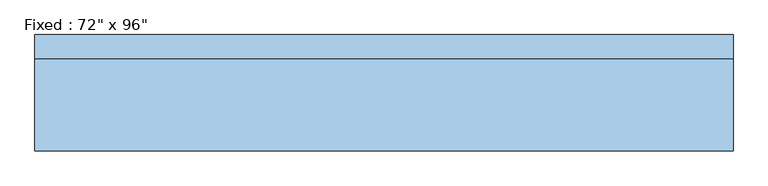
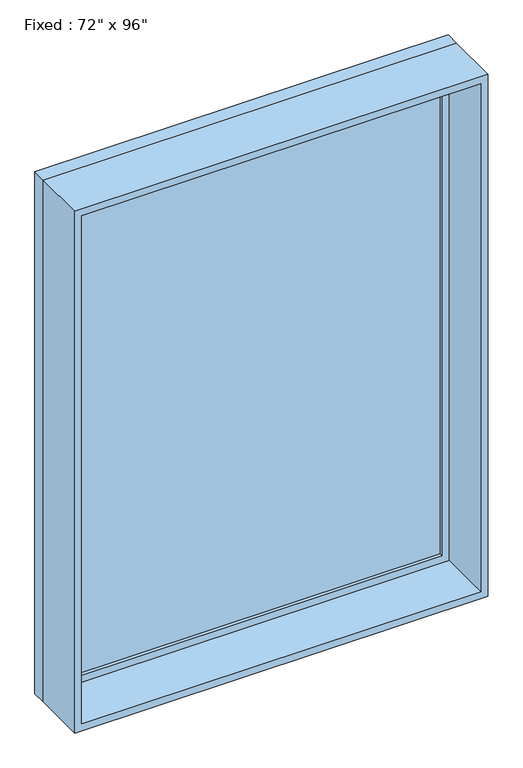
"""IFC4 building model written with IfcOpenShell, lengths in millimetres: window geometry."""

from ifc_helpers import new_model, si_unit, frame, origin, place, context, project, spatial, polyline, outline, extrude, source, transform, mapped, element, save


def window_1de08d8e(model_context):
    return source(origin(), model_context, "Body", "SweptSolid", [
        extrude(outline(polyline([(812.8, 104.775), (-889.0, 104.775), (-889.0, 117.475), (812.8, 117.475), (812.8, 104.775)])), frame((0.0, 0.0, 368.3), z_axis=(0.0, 0.0, 1.0), x_axis=(1.0, 0.0, 0.0)), (0.0, 0.0, 1.0), 2311.4),
        extrude(outline(polyline([(2724.15, -933.45), (323.85, -933.45), (323.85, 857.25), (2724.15, 857.25), (2724.15, -933.45)]), holes=[polyline([(2679.7, -889.0), (2679.7, 812.8), (368.3, 812.8), (368.3, -889.0), (2679.7, -889.0)])]), frame((0.0, 88.9, 0.0), z_axis=(0.0, 1.0, 0.0), x_axis=(0.0, 0.0, 1.0)), (0.0, 0.0, 1.0), 44.45),
        extrude(outline(polyline([(2743.2, -952.5), (304.8, -952.5), (304.8, 876.3), (2743.2, 876.3), (2743.2, -952.5)]), holes=[polyline([(2711.45, -920.75), (2711.45, 844.55), (336.55, 844.55), (336.55, -920.75), (2711.45, -920.75)])]), frame((0.0, -152.4, 0.0), z_axis=(0.0, 1.0, 0.0), x_axis=(0.0, 0.0, 1.0)), (0.0, 0.0, 1.0), 241.3),
        extrude(outline(polyline([(2743.2, 876.3), (2743.2, -952.5), (304.8, -952.5), (304.8, 876.3), (2743.2, 876.3)]), holes=[polyline([(2724.15, 857.25), (323.85, 857.25), (323.85, -933.45), (2724.15, -933.45), (2724.15, 857.25)])]), frame((0.0, 88.9, 0.0), z_axis=(0.0, 1.0, 0.0), x_axis=(0.0, 0.0, 1.0)), (0.0, 0.0, 1.0), 63.5),
    ])


if __name__ == "__main__":
    model = new_model("IFC4")
    model_context = context("Model", 3, world=origin())
    ifc_project = project(units=[si_unit("LENGTHUNIT", "METRE", prefix="MILLI")], contexts=[model_context])
    site = spatial("IfcSite", under=ifc_project)
    building = spatial("IfcBuilding", under=site)
    placement = place(None, origin())
    window_shape = window_1de08d8e(model_context)
    element("IfcWindow", 1, ObjectType="Fixed : 72\" x 96\"", at=placement, inside=building, context=model_context, shape_type="MappedRepresentation", body=[
        mapped(window_shape, transform((0.0, 0.0, 0.0), x_axis=(1.0, 0.0, 0.0), y_axis=(0.0, 1.0, 0.0), z_axis=(0.0, 0.0, 1.0))),
    ])
    save(model, "model.ifc")

# Revit data of these elements
# Type "Fixed : 72\" x 96\""
#   Type Mark = "11"
#   Construction Type Id = "GSP4R"
#   Assembly Code = "B2020100"
#   Analytic Construction = "1/8 in Pilkington single glazing"
#   Visual Light Transmittance = 0.9
#   Solar Heat Gain Coefficient = 0.78
#   Heat Transfer Coefficient (U) = 0.6496 BTU/(h·ft²·°F)
#   Height = 8' - 0"
#   Default Sill Height = 1' - 0"
#   Width = 6' - 0"
#   Window Inset = 0' - 0 3/4"
#   Define Thermal Properties by = 1
#   Glass Pane Material = Glass
#   Sash Material = Iron, Ductile
#   Wall Closure = (empty or 0)
# Element 1 (IfcWindow, "Fixed : 72\" x 96\"")
#   Materials on its faces: "Iron, Ductile", "Glass"
# Materials
#   "Glass": class "Glass", colour RGB 0 128 192, transparency 0.75, Description = "Soda Lime Glass", Cost = 0
#   "Iron, Ductile": class "Metal", colour RGB 0 0 0, transparency 0, Description = "Ductile cast iron", Cost = 0
